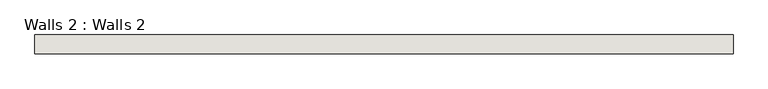
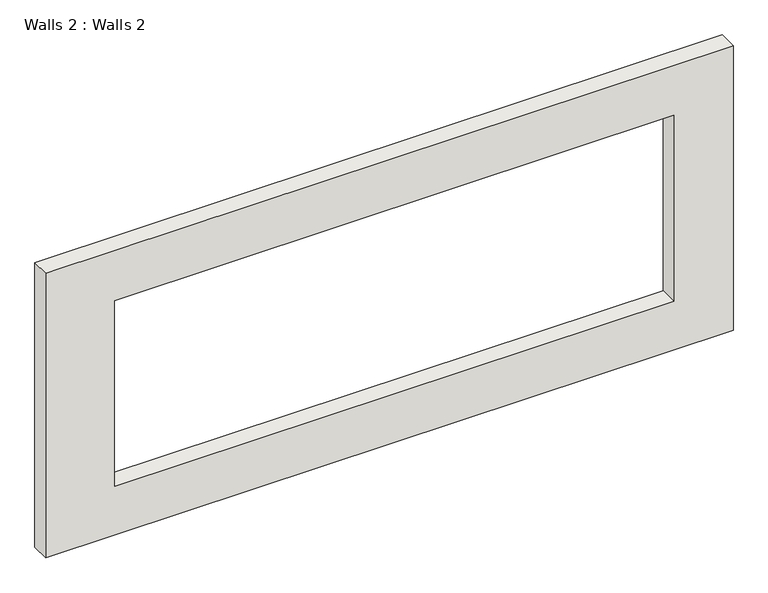
"""IFC4 building model written with IfcOpenShell, lengths in millimetres: wall geometry, Walls 2 : Walls 2."""

from ifc_helpers import new_model, si_unit, frame, origin, place, context, project, spatial, polyline, outline, extrude, source, transform, mapped, element, save


def walls_2_walls_2_aacfb59a(model_context):
    return source(origin(), model_context, "Body", "SweptSolid", [
        extrude(outline(polyline([(3973.3839769, -11535.2764802), (3973.3839769, -3925.6745124), (7302.5, -3925.6745124), (7302.5, -11535.2764802), (3973.3839769, -11535.2764802)]), holes=[polyline([(6714.4549819, -4580.8162469), (4540.5031698, -4580.8162469), (4540.5031698, -10772.9605216), (6714.4549819, -10772.9605216), (6714.4549819, -4580.8162469)])]), frame((0.0, -833.9390518, 0.0), z_axis=(0.0, 1.0, 0.0), x_axis=(0.0, 0.0, 1.0)), (0.0, 0.0, 1.0), 206.2125023),
    ])


if __name__ == "__main__":
    model = new_model("IFC4")
    model_context = context("Model", 3, world=origin())
    ifc_project = project(units=[si_unit("LENGTHUNIT", "METRE", prefix="MILLI")], contexts=[model_context])
    site = spatial("IfcSite", under=ifc_project)
    building = spatial("IfcBuilding", under=site)
    placement = place(None, origin())
    walls_2_walls_2_shape = walls_2_walls_2_aacfb59a(model_context)
    element("IfcWall", 1, ObjectType="Walls 2 : Walls 2", at=placement, inside=building, context=model_context, shape_type="MappedRepresentation", body=[
        mapped(walls_2_walls_2_shape, transform((0.0, 0.0, 0.0), x_axis=(1.0, 0.0, 0.0), y_axis=(0.0, 1.0, 0.0), z_axis=(0.0, 0.0, 1.0))),
    ])
    save(model, "model.ifc")

# Revit data of these elements
# Element 1 (IfcWall, "Walls 2 : Walls 2")
#   Materials on its faces: "Default Wall"
# Materials
#   "Default Wall": colour RGB 128 128 128, transparency 0
